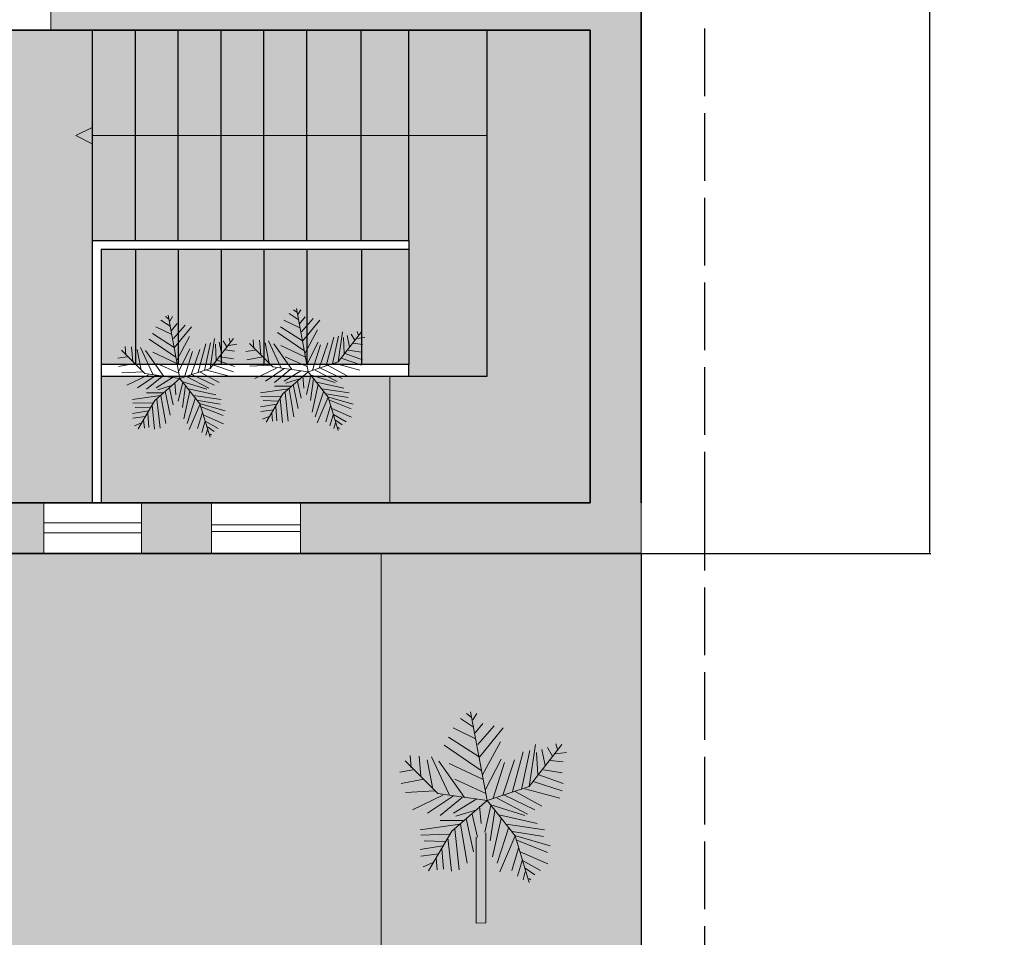
# Model space of a CAD drawing. Units: inches. Extents: x 1316 to 1777, y 813 to 1650.
# Tile 4 of 22: x 1603 to 1777, y 963 to 1126. Entities that reach past the tile are written whole.
import ezdxf

# ---------------------------------------------------------------- set-up
doc = ezdxf.new("R2010")
doc.units = ezdxf.units.IN
doc.header["$MEASUREMENT"] = 0
doc.linetypes.add('ACAD_ISO02W100', pattern=[15, 12, -3])
for name, color, linetype, lineweight in [('A-ANNO-DIMS', 2, 'Continuous', 18), ('A-ANNO-SYMB', 7, 'Continuous', 18), ('A-ANNO-SYMB-PATT', 7, 'Continuous', 13), ('A-FLOR-STRS', 7, 'Continuous', 25), ('A-FLOR-STRS-PATT', 252, 'Continuous', 13), ('A-WALL-PATT', 250, 'Continuous', 13), ('C-PROP', 8, 'ACAD_ISO02W100', 25), ('greenary', 106, 'Continuous', 13), ('L-HRDS', 8, 'Continuous', 18), ('L-HRDS-PATT', 252, 'Continuous', 13), ('L-PLNT-PATT', 74, 'Continuous', 13), ('walls', 250, 'Continuous', 35), ('windows', 141, 'Continuous', 18)]:
    doc.layers.add(name, color=color, linetype=linetype, lineweight=lineweight)
doc.layers.add('A-FLOR-PATT', color=254, linetype='Continuous', lineweight=13, true_color=0xfeeab9)
doc.styles.get("Standard").update_dxf_attribs({"font": 'arial.ttf'})
doc.dimstyles.get("Standard").update_dxf_attribs({"dimtxt": 7, "dimasz": 0.18, "dimexe": 0.18, "dimexo": 0.0625, "dimgap": 0.09, "dimtad": 0, "dimtih": 1, "dimtoh": 1, "dimzin": 0, "dimdsep": 46, "dimlunit": 3, "dimtxsty": 'Standard', "dimcen": 0.09, "dimadec": 0, "dimazin": 0, "dimtfac": 1, "dimtofl": 0, "dimtmove": 0, "dimatfit": 3, "dimfxl": 1, "dimtolj": 1, "dimtzin": 0, "dimarcsym": 0})

# ---------------------------------------------------------------- blocks, each defined once
blk = doc.blocks.new('*U13')
for p, q in [((0, 0), (-10.5, 57)), ((-8.737, 47.138), (-17.069, 52.711)), ((-10.186, 53.64), (-13.084, 55.962)), ((-9.099, 51.782), (-6.563, 55.962)), ((-7.288, 39.707), (-21.778, 46.673)), ((-7.65, 43.423), (-2.578, 49.46)), ((-5.839, 35.992), (4.667, 48.067)), ((-5.114, 27.632), (10.463, 46.673)), ((-5.114, 28.097), (-24.676, 40.636)), ((-3.665, 19.273), (-27.574, 35.527)), ((-2.941, 16.486), (8.652, 37.85)), ((22.055, 7.198), (27.489, 32.277)), ((27, 9), (48, 36)), ((27.127, 9.056), (31.112, 35.992)), ((35.096, 32.741), (37.27, 22.524)), ((38.719, 34.134), (41.979, 28.561)), ((44.153, 36.456), (45.239, 32.741)), ((-31.5, 4.5), (-52.5, 25.5)), ((-48.585, 21.131), (-49.309, 29.026)), ((-43.513, 28.561), (-42.427, 15.558)), ((-38.442, 26.239), (-34.819, 7.663)), ((-35.544, 28.097), (-24.314, 3.947)), ((-14.533, 2.09), (-30.834, 25.31)), ((-1.129, 6.734), (9.014, 26.704)), ((10.101, 3.483), (17.708, 26.239)), ((16.259, 5.805), (23.142, 31.348)), ((31.836, 30.883), (32.561, 16.486)), ((40.53, 25.775), (48.862, 24.846)), ((43.791, 29.954), (51.036, 30.883)), ((-47.498, 19.737), (-55.83, 18.344)), ((-24.314, 23.917), (-2.941, 13.7)), ((3.942, 1.625), (11.187, 24.381)), ((36.183, 19.737), (48.137, 17.88)), ((-40.615, 13.7), (-55.105, 10.913)), ((-20.691, 13.7), (-1.129, 4.876)), ((33.285, 16.486), (48.862, 10.913)), ((0, 0), (27, 9)), ((24.229, 7.663), (46.688, 1.625)), ((29.662, 12.307), (48.137, 6.269)), ((-33.37, 6.269), (-52.207, 5.34)), ((-28.299, 3.483), (-47.86, -5.805)), ((-21.416, 3.018), (-38.079, -8.128)), ((0, 0), (-31.5, 4.5)), ((-15.982, 2.09), (-30.11, -9.521)), ((0, 0), (-22.5, -19.5)), ((-6.563, 1.161), (-21.416, -8.128)), ((0, 0), (18, -22.5)), ((6.478, 1.625), (26.04, -8.592)), ((11.187, 3.483), (30.749, -5.805)), ((18.07, 5.805), (35.096, -3.483)), ((-6.563, -5.805), (-19.967, -9.985)), ((-4.752, -3.483), (-3.665, -14.629)), ((2.493, -3.019), (-1.491, -20.202)), ((1.769, -2.555), (24.229, -9.521)), ((5.029, -6.27), (2.131, -25.775)), ((-13.446, -11.378), (-8.737, -32.741)), ((-9.461, -8.592), (-6.201, -23.453)), ((9.014, -11.378), (3.58, -35.992)), ((7.565, -9.056), (32.198, -14.629)), ((-17.431, -15.094), (-42.789, -18.809)), ((-15.257, -12.772), (-30.11, -12.772)), ((-20.691, -18.345), (-17.793, -44.352)), ((-17.069, -15.094), (-12.721, -40.172)), ((14.085, -16.951), (6.478, -40.172)), ((12.274, -15.094), (36.907, -18.809)), ((-24.314, -21.596), (-42.427, -22.06)), ((-22.5, -19.5), (-37.5, -45)), ((-25.038, -23.918), (-22.865, -45.281)), ((18.07, -22.524), (8.289, -45.745)), ((16.259, -19.738), (36.183, -22.989)), ((18, -22.5), (27, -52.5)), ((18.433, -22.524), (40.53, -29.026)), ((-28.299, -29.026), (-42.789, -31.348)), ((-26.849, -26.24), (-40.253, -25.775)), ((-29.023, -30.884), (-27.936, -43.887)), ((20.244, -30.419), (15.897, -44.816)), ((19.157, -25.311), (38.719, -33.206)), ((-30.834, -34.135), (-42.427, -35.528)), ((-32.646, -36.921), (-31.921, -44.352)), ((22.78, -37.85), (19.519, -48.532)), ((21.331, -32.741), (39.081, -40.636)), ((-34.457, -39.708), (-40.978, -42.494)), ((22.78, -38.314), (34.372, -44.816)), ((24.591, -43.423), (30.749, -47.603)), ((24.591, -45.745), (23.142, -50.854)), ((26.764, -49.925), (28.213, -50.854))]:
    blk.add_line(p, q)
blk = doc.blocks.new('*D50')
at = {"layer": 'A-ANNO-DIMS', "color": 0, "lineweight": -2, "transparency": 16777216}
for p, q in [((1377.06, 1063.81), (1377.06, 817.77)), ((1713.17, 1031.11), (1713.17, 817.77)), ((1377.24, 817.95), (1532.95, 817.95)), ((1712.99, 817.95), (1557.29, 817.95))]:
    blk.add_line(p, q, dxfattribs=at)
at = {"layer": 'A-ANNO-DIMS', "color": 0, "transparency": 16777216}
for points in [[(1377.24, 817.98), (1377.24, 817.92), (1377.06, 817.95)], [(1712.99, 817.98), (1712.99, 817.92), (1713.17, 817.95)]]:
    blk.add_solid(points, dxfattribs=at)
at = {"layer": 'Defpoints', "color": 0, "transparency": 16777216}
for p in [(1377.06, 1063.87), (1713.17, 1031.17), (1713.17, 817.95)]:
    blk.add_point(p, dxfattribs=at)
at = {"layer": 'A-ANNO-DIMS', "color": 0, "transparency": 16777216, "insert": (1545.12, 817.95), "char_height": 7, "attachment_point": 5}
blk.add_mtext('\\A1;28\'-0"', dxfattribs=at)
blk = doc.blocks.new('*D51')
at = {"layer": 'A-ANNO-DIMS', "color": 0, "lineweight": -2, "transparency": 16777216}
for p, q in [((1713.24, 1575.37), (1764.48, 1575.37)), ((1764.3, 1575.19), (1764.3, 1306.92)), ((1764.3, 1031.35), (1764.3, 1299.62)), ((1713.24, 1031.17), (1764.48, 1031.17))]:
    blk.add_line(p, q, dxfattribs=at)
at = {"layer": 'A-ANNO-DIMS', "color": 0, "transparency": 16777216}
for points in [[(1764.27, 1575.19), (1764.33, 1575.19), (1764.3, 1575.37)], [(1764.27, 1031.35), (1764.33, 1031.35), (1764.3, 1031.17)]]:
    blk.add_solid(points, dxfattribs=at)
at = {"layer": 'Defpoints', "color": 0, "transparency": 16777216}
for p in [(1713.17, 1575.37), (1764.3, 1575.37), (1713.17, 1031.17)]:
    blk.add_point(p, dxfattribs=at)
at = {"layer": 'A-ANNO-DIMS', "color": 0, "transparency": 16777216, "insert": (1764.3, 1303.27), "char_height": 7, "attachment_point": 5}
blk.add_mtext('\\A1;45\'-4"', dxfattribs=at)

msp = doc.modelspace()

# ---------------------------------------------------------------- hatches: boundary and pattern name
at = {"layer": 'A-ANNO-SYMB-PATT'}
h = msp.add_hatch(color=256, dxfattribs=at)
h.dxf.hatch_style = 1
h.paths.add_polyline_path([(1613.066, 1105.235), (1616.06, 1103.693), (1616.06, 1105.253), (1616.06, 1106.696)])
at = {"layer": 'A-FLOR-PATT'}
h = msp.add_hatch(color=256, dxfattribs=at)
h.dxf.hatch_style = 1
h.paths.add_polyline_path([(1567.673, 1281.369), (1651.673, 1281.369), (1651.673, 1365.369), (1597.673, 1365.369), (1597.673, 1429.869), (1570.345, 1429.869), (1570.345, 1471.869), (1510.345, 1471.869), (1510.345, 1429.869), (1444.564, 1429.869), (1444.564, 1322.882), (1444.564, 1300.088), (1510.564, 1300.088), (1510.564, 1295.094), (1510.564, 1240.869), (1386.064, 1240.869), (1386.064, 1171.185), (1400.961, 1171.185), (1400.961, 1106.742), (1386.064, 1106.742), (1386.064, 1072.869), (1510.564, 1072.869), (1510.564, 1040.173), (1541.068, 1040.173, -0.367085), (1572.764, 1069.547), (1572.764, 1069.579), (1574.225, 1069.579), (1574.225, 1040.173), (1616.037, 1040.173), (1616.037, 1086.627), (1616.037, 1103.705), (1613.066, 1105.235), (1616.037, 1106.686), (1616.037, 1123.869), (1567.673, 1123.869)])
h.paths.add_polyline_path([(1508.987, 1198.018), (1511.117, 1198.018), (1511.117, 1200.148), (1532.595, 1200.148), (1532.595, 1198.018), (1534.725, 1198.018), (1534.725, 1176.008), (1530.465, 1176.008), (1530.465, 1176.718), (1513.247, 1176.718), (1513.247, 1176.008), (1508.987, 1176.008)], flags=16)
h.paths.add_polyline_path([(1505.979, 1151.315), (1521.504, 1151.315), (1521.504, 1123.623), (1505.979, 1123.623)], flags=16)
h.paths.add_polyline_path([(1507.734, 1150.101, -1), (1506.932, 1150.101, -1)], flags=0)
h.paths.add_polyline_path([(1512.288, 1138.353), (1512.28, 1138.392), (1512.219, 1138.376)], flags=0)
h.paths.add_polyline_path([(1511.539, 1138.926), (1511.802, 1138.967), (1511.817, 1139.27), (1511.607, 1139.246)], flags=0)
h.paths.add_polyline_path([(1513.745, 1140.234), (1513.68, 1139.885), (1514.014, 1140.045), (1513.855, 1140.308)], flags=0)
h.paths.add_polyline_path([(1513.759, 1139.089), (1514.005, 1139.255), (1513.807, 1139.483), (1513.564, 1139.327)], flags=0)
h.paths.add_polyline_path([(1514.219, 1138.385), (1514.336, 1138.33), (1514.544, 1138.32), (1514.802, 1138.874), (1514.451, 1138.716)], flags=0)
h.paths.add_polyline_path([(1514.577, 1137.439), (1514.573, 1137.4), (1514.699, 1137.4), (1514.696, 1137.402)], flags=0)
h.paths.add_polyline_path([(1512.26, 1136.199), (1512.199, 1136.399), (1512.032, 1136.325), (1512.095, 1136.101), (1512.257, 1136.192)], flags=0)
h.paths.add_polyline_path([(1512.644, 1137.274), (1512.356, 1137.23), (1512.432, 1137.049), (1512.703, 1137.093)], flags=0)
h.paths.add_polyline_path([(1513.049, 1137.593), (1512.979, 1137.8), (1512.843, 1137.757), (1512.887, 1137.556)], flags=0)
h.paths.add_polyline_path([(1513.269, 1138.556), (1513.571, 1137.962), (1513.459, 1136.814), (1513.212, 1137.878), (1513.032, 1138.443)], flags=0)
h.paths.add_polyline_path([(1514.891, 1136.377), (1514.696, 1136.401), (1514.683, 1136.246), (1514.87, 1136.165)], flags=0)
h.paths.add_polyline_path([(1514.142, 1137.293), (1514.047, 1136.743), (1514.27, 1136.751), (1514.328, 1137.265)], flags=0)
h.paths.add_polyline_path([(1515.362, 1138.976), (1515.334, 1138.638), (1515.596, 1138.588), (1515.627, 1138.932)], flags=0)
h.paths.add_polyline_path([(1537.285, 1177.912), (1537.995, 1177.912), (1537.995, 1195.13), (1537.285, 1195.13), (1537.285, 1199.39), (1559.295, 1199.39), (1559.295, 1197.26), (1561.425, 1197.26), (1561.425, 1175.782), (1559.295, 1175.782), (1559.295, 1173.652), (1559.379, 1173.652), (1559.379, 1171.514), (1561.517, 1171.514), (1561.517, 1098.819), (1559.379, 1098.819), (1559.379, 1096.68), (1537.285, 1096.68), (1537.285, 1100.957), (1537.997, 1100.957), (1537.997, 1169.376), (1537.285, 1169.376), (1537.285, 1173.652)], flags=16)
h.paths.add_polyline_path([(1518.623, 1345.565), (1519.133, 1345.48), (1519.133, 1345.485), (1518.623, 1345.567)], flags=16)
h.paths.add_polyline_path([(1518.798, 1374.15), (1519.308, 1374.064), (1519.308, 1374.069), (1518.798, 1374.152)], flags=16)
h.paths.add_polyline_path([(1537.764, 1413.501), (1537.678, 1412.991), (1537.683, 1412.991), (1537.766, 1413.501)], flags=16)
h.paths.add_polyline_path([(1572.905, 1373.821), (1573.927, 1373.975), (1574.027, 1390.309), (1573.007, 1390.475), (1573.007, 1390.475)], flags=16)
h.paths.add_polyline_path([(1572.73, 1345.237), (1573.752, 1345.39), (1573.852, 1361.724), (1572.832, 1361.89), (1572.832, 1361.89)], flags=16)
h.paths.add_polyline_path([(1537.211, 1322.643), (1537.364, 1321.621), (1553.698, 1321.521), (1553.864, 1322.541)], flags=16)
h.paths.add_polyline_path([(1535.908, 1331.328), (1527.214, 1331.382), (1527.664, 1404.885), (1564.416, 1404.66), (1563.966, 1331.157), (1555.273, 1331.21), (1553.947, 1323.051), (1537.134, 1323.154)], flags=16)
h.paths.add_polyline_path([(1536.15, 1336.503), (1536.235, 1337.572), (1536.323, 1338.628), (1536.411, 1339.663), (1536.495, 1340.67), (1536.574, 1341.66), (1536.648, 1342.648), (1536.717, 1343.649), (1536.78, 1344.678), (1536.837, 1345.75), (1536.913, 1347.475), (1536.93, 1348.082), (1536.867, 1346.314), (1536.754, 1344.188), (1536.619, 1342.219), (1536.495, 1340.67), (1536.411, 1339.663), (1536.323, 1338.628), (1536.235, 1337.572), (1536.15, 1336.503), (1536.071, 1335.432), (1536.002, 1334.37), (1535.917, 1332.754), (1535.909, 1332.308), (1535.964, 1333.78), (1536.071, 1335.432)], flags=0)
h.paths.add_polyline_path([(1540.412, 1338.345), (1540.539, 1339.037), (1540.667, 1339.758), (1540.798, 1340.518), (1540.93, 1341.325), (1541.063, 1342.187), (1541.196, 1343.109), (1541.326, 1344.085), (1541.45, 1345.102), (1541.566, 1346.15), (1541.669, 1347.219), (1541.758, 1348.296), (1541.829, 1349.371), (1541.879, 1350.434), (1541.906, 1351.476), (1541.91, 1352.5), (1541.895, 1353.512), (1541.861, 1354.518), (1541.812, 1355.524), (1541.749, 1356.537), (1541.674, 1357.561), (1541.551, 1359.062), (1541.495, 1359.67), (1541.589, 1358.603), (1541.721, 1356.977), (1541.846, 1354.98), (1541.912, 1352.982), (1541.903, 1350.951), (1541.806, 1348.87), (1541.628, 1346.713), (1541.396, 1344.612), (1541.135, 1342.656), (1540.872, 1340.947), (1540.617, 1339.466), (1540.412, 1338.345), (1540.288, 1337.675), (1540.166, 1337.018), (1540.049, 1336.365), (1539.937, 1335.71), (1539.837, 1335.055), (1539.758, 1334.403), (1539.709, 1333.756), (1539.697, 1333.12), (1539.751, 1332.162), (1539.822, 1331.89), (1539.691, 1332.775), (1539.714, 1334.035), (1539.867, 1335.303), (1540.085, 1336.577), (1540.288, 1337.675)], flags=0)
h.paths.add_polyline_path([(1545.599, 1331.584), (1545.601, 1331.617), (1545.614, 1331.689), (1545.737, 1332.197), (1545.767, 1332.332), (1545.84, 1332.681), (1545.925, 1333.114), (1546.016, 1333.614), (1546.108, 1334.164), (1546.196, 1334.748), (1546.276, 1335.349), (1546.342, 1335.952), (1546.388, 1336.539), (1546.412, 1337.098), (1546.414, 1337.632), (1546.395, 1338.145), (1546.359, 1338.645), (1546.306, 1339.137), (1546.24, 1339.627), (1546.161, 1340.121), (1546.073, 1340.625), (1545.888, 1341.63), (1545.718, 1342.621), (1545.547, 1343.945), (1545.432, 1345.534), (1545.404, 1347.402), (1545.418, 1348.013), (1545.411, 1346.957), (1545.425, 1345.988), (1545.463, 1345.105), (1545.521, 1344.301), (1545.596, 1343.566), (1545.683, 1342.892), (1545.778, 1342.27), (1545.877, 1341.691), (1545.977, 1341.145), (1546.133, 1340.297), (1546.327, 1339.075), (1546.434, 1337.615), (1546.377, 1336.279), (1546.246, 1335.079), (1546.032, 1333.665), (1545.84, 1332.681), (1545.767, 1332.332)], flags=0)
h.paths.add_polyline_path([(1551.803, 1337.656), (1551.963, 1338.25), (1552.102, 1338.801), (1552.225, 1339.338), (1552.331, 1339.865), (1552.418, 1340.377), (1552.487, 1340.873), (1552.536, 1341.348), (1552.563, 1341.801), (1552.569, 1342.228), (1552.551, 1342.627), (1552.51, 1342.995), (1552.446, 1343.333), (1552.363, 1343.646), (1552.261, 1343.937), (1552.144, 1344.207), (1552.012, 1344.461), (1551.868, 1344.7), (1551.746, 1344.882), (1550.887, 1346.052), (1550.428, 1347.126), (1550.183, 1348.353), (1550.048, 1349.632), (1549.978, 1351.224), (1549.974, 1353.141), (1549.989, 1353.748), (1549.975, 1352.682), (1549.977, 1351.708), (1549.996, 1350.825), (1550.031, 1350.027), (1550.082, 1349.31), (1550.15, 1348.669), (1550.234, 1348.098), (1550.335, 1347.593), (1550.452, 1347.149), (1550.584, 1346.76), (1550.73, 1346.419), (1550.887, 1346.117), (1551.05, 1345.848), (1551.217, 1345.602), (1551.386, 1345.372), (1551.553, 1345.151), (1552, 1344.537), (1552.454, 1343.495), (1552.591, 1342.266), (1552.509, 1340.905), (1552.246, 1339.367), (1551.925, 1338.101), (1551.619, 1336.984), (1551.406, 1336.2), (1551.01, 1334.699), (1550.877, 1334.155), (1551.264, 1335.677), (1551.619, 1336.984)], flags=0)
h.paths.add_polyline_path([(1558.642, 1348.348), (1558.795, 1348.811), (1558.918, 1349.215), (1559.008, 1349.575), (1559.061, 1349.904), (1559.076, 1350.214), (1559.054, 1350.506), (1559.001, 1350.776), (1558.919, 1351.021), (1558.814, 1351.239), (1558.688, 1351.425), (1558.546, 1351.578), (1558.392, 1351.694), (1558.229, 1351.772), (1558.059, 1351.812), (1557.882, 1351.819), (1557.701, 1351.794), (1557.515, 1351.742), (1557.327, 1351.665), (1557.136, 1351.566), (1556.944, 1351.448), (1556.752, 1351.315), (1556.742, 1351.307), (1556.175, 1350.878), (1555.982, 1350.741), (1555.79, 1350.618), (1555.103, 1350.248), (1554.019, 1350.696), (1553.658, 1351.734), (1553.592, 1352.861), (1553.705, 1354.248), (1553.753, 1354.657), (1553.685, 1354.004), (1553.638, 1353.425), (1553.615, 1352.918), (1553.615, 1352.476), (1553.637, 1352.094), (1553.681, 1351.766), (1553.745, 1351.485), (1553.828, 1351.246), (1553.929, 1351.043), (1554.048, 1350.87), (1554.182, 1350.722), (1554.33, 1350.599), (1554.491, 1350.501), (1554.662, 1350.43), (1554.841, 1350.388), (1555.026, 1350.374), (1555.215, 1350.39), (1555.406, 1350.437), (1555.598, 1350.514), (1555.79, 1350.618), (1555.982, 1350.741), (1556.175, 1350.878), (1556.367, 1351.024), (1556.559, 1351.171), (1556.752, 1351.315), (1556.944, 1351.448), (1557.136, 1351.566), (1557.327, 1351.665), (1558.043, 1351.957), (1558.894, 1351.316), (1559.137, 1350.09), (1558.886, 1349.087), (1558.642, 1348.348), (1558.463, 1347.812), (1558.261, 1347.187), (1558.039, 1346.459), (1557.677, 1345.175), (1557.549, 1344.636), (1557.909, 1346.03), (1558.329, 1347.408)], flags=0)
h.paths.add_polyline_path([(1562.145, 1353.919), (1562.25, 1354.68), (1562.341, 1355.344), (1562.416, 1355.924), (1562.475, 1356.431), (1562.518, 1356.872), (1562.544, 1357.254), (1562.554, 1357.582), (1562.548, 1357.862), (1562.525, 1358.1), (1562.486, 1358.303), (1562.432, 1358.476), (1562.361, 1358.624), (1562.277, 1358.748), (1562.18, 1358.848), (1562.073, 1358.925), (1561.958, 1358.977), (1561.837, 1359.006), (1561.711, 1359.011), (1561.584, 1358.992), (1561.456, 1358.949), (1561.342, 1358.895), (1560.78, 1358.554), (1560.631, 1358.473), (1560.474, 1358.403), (1560.311, 1358.348), (1559.637, 1358.207), (1558.973, 1358.904), (1558.816, 1360.002), (1558.804, 1361.236), (1558.83, 1361.674), (1558.807, 1360.917), (1558.813, 1360.297), (1558.845, 1359.795), (1558.902, 1359.397), (1558.982, 1359.087), (1559.082, 1358.849), (1559.2, 1358.666), (1559.334, 1358.525), (1559.482, 1358.421), (1559.639, 1358.351), (1559.804, 1358.311), (1559.973, 1358.3), (1560.143, 1358.313), (1560.311, 1358.348), (1560.474, 1358.403), (1560.631, 1358.473), (1560.78, 1358.554), (1560.923, 1358.641), (1561.061, 1358.729), (1561.196, 1358.813), (1561.382, 1358.92), (1561.342, 1358.895), (1561.972, 1359.194), (1562.536, 1358.367), (1562.56, 1357.311), (1562.455, 1356.226), (1562.323, 1355.206), (1562.145, 1353.919), (1562.026, 1353.049), (1561.815, 1351.457), (1561.752, 1350.933), (1561.948, 1352.479)], flags=0)
h.paths.add_polyline_path([(1572.764, 1069.547, 0.367085), (1541.068, 1040.173), (1572.764, 1040.173)], flags=17)
h.paths.add_polyline_path([(1572.764, 1040.173), (1541.068, 1040.173, 0.0299535), (1540.829, 1036.182), (1540.829, 1031.173), (1574.225, 1031.173), (1574.225, 1036.182), (1572.764, 1036.182)])
at = {"layer": 'A-FLOR-STRS-PATT'}
h = msp.add_hatch(color=256, dxfattribs=at)
h.dxf.hatch_style = 1
h.paths.add_polyline_path([(1623.621, 1105.248), (1616.037, 1105.248), (1616.037, 1086.627), (1623.621, 1086.627)])
h.paths.add_polyline_path([(1623.621, 1123.869), (1616.037, 1123.869), (1616.037, 1105.248), (1623.621, 1105.248)])
h.paths.add_polyline_path([(1631.206, 1105.248), (1623.621, 1105.248), (1623.621, 1086.627), (1631.206, 1086.627)])
h.paths.add_polyline_path([(1631.206, 1123.869), (1623.621, 1123.869), (1623.621, 1105.248), (1631.206, 1105.248)])
h.paths.add_polyline_path([(1638.79, 1105.248), (1631.206, 1105.248), (1631.206, 1086.627), (1638.79, 1086.627)])
h.paths.add_polyline_path([(1638.79, 1123.869), (1631.206, 1123.869), (1631.206, 1105.248), (1638.79, 1105.248)])
h.paths.add_polyline_path([(1646.374, 1105.248), (1638.79, 1105.248), (1638.79, 1086.627), (1646.374, 1086.627)])
h.paths.add_polyline_path([(1646.374, 1123.869), (1638.79, 1123.869), (1638.79, 1105.248), (1646.374, 1105.248)])
h.paths.add_polyline_path([(1653.958, 1105.248), (1646.374, 1105.248), (1646.374, 1086.627), (1653.958, 1086.627)])
h.paths.add_polyline_path([(1653.958, 1123.869), (1646.374, 1123.869), (1646.374, 1105.248), (1653.958, 1105.248)])
h.paths.add_polyline_path([(1663.586, 1105.248), (1653.958, 1105.248), (1653.958, 1086.627), (1663.586, 1086.627)])
h.paths.add_polyline_path([(1663.586, 1123.869), (1653.958, 1123.869), (1653.958, 1105.248), (1663.586, 1105.248)])
h.paths.add_polyline_path([(1672.026, 1105.248), (1663.586, 1105.248), (1663.586, 1086.627), (1672.026, 1086.627)])
h.paths.add_polyline_path([(1672.026, 1123.869), (1663.586, 1123.869), (1663.586, 1105.248), (1672.026, 1105.248)])
h = msp.add_hatch(color=256, dxfattribs=at)
h.dxf.hatch_style = 1
h.paths.add_polyline_path([(1685.903, 1105.248), (1672.026, 1105.248), (1672.026, 1086.627), (1672.026, 1085.053), (1672.026, 1064.656), (1672.026, 1062.613), (1685.903, 1062.613)])
h.paths.add_polyline_path([(1685.903, 1123.869), (1672.026, 1123.869), (1672.026, 1105.248), (1685.903, 1105.248)])
h = msp.add_hatch(color=256, dxfattribs=at)
h.dxf.hatch_style = 1
h.paths.add_polyline_path([(1623.621, 1085.053), (1617.549, 1085.053), (1617.549, 1064.656), (1623.621, 1064.656)])
h.paths.add_polyline_path([(1631.206, 1085.053), (1623.621, 1085.053), (1623.621, 1064.656), (1631.206, 1064.656)])
h.paths.add_polyline_path([(1638.79, 1085.053), (1631.206, 1085.053), (1631.206, 1064.656), (1638.79, 1064.656)])
h.paths.add_polyline_path([(1646.374, 1085.053), (1638.79, 1085.053), (1638.79, 1064.656), (1646.374, 1064.656)])
h.paths.add_polyline_path([(1653.958, 1085.053), (1646.374, 1085.053), (1646.374, 1064.656), (1653.958, 1064.656)])
h.paths.add_polyline_path([(1663.648, 1085.053), (1653.958, 1085.053), (1653.958, 1064.656), (1663.648, 1064.656)])
h.paths.add_polyline_path([(1672.026, 1085.053), (1663.648, 1085.053), (1663.648, 1064.656), (1672.026, 1064.656)])
at = {"layer": 'A-WALL-PATT'}
h = msp.add_hatch(color=256, dxfattribs=at)
h.dxf.hatch_style = 1
h.paths.add_polyline_path([(1713.173, 1281.369), (1656.173, 1281.369), (1656.173, 1298.258), (1651.673, 1298.258), (1651.673, 1281.369), (1567.673, 1281.369), (1567.673, 1266.995), (1572.173, 1266.995), (1572.173, 1276.869), (1704.173, 1276.869), (1704.173, 1132.869), (1608.64, 1132.869), (1608.64, 1123.869), (1704.173, 1123.869), (1704.173, 1040.173), (1652.869, 1040.173), (1652.869, 1031.173), (1713.173, 1031.173), (1713.173, 1040.173)])
h.paths.add_polyline_path([(1572.173, 1237.955), (1567.673, 1237.955), (1567.673, 1123.869), (1583.146, 1123.869), (1583.146, 1132.869), (1572.173, 1132.869)], flags=17)
h.paths.add_polyline_path([(1510.345, 1566.369), (1524.171, 1566.369), (1524.171, 1571.985), (1524.171, 1575.369), (1445.955, 1575.369), (1445.955, 1566.369), (1505.845, 1566.369), (1505.845, 1469.591), (1510.345, 1469.591), (1510.345, 1471.869), (1529.081, 1471.869), (1529.081, 1476.369), (1510.345, 1476.369)])
h.paths.add_polyline_path([(1609.722, 1575.369), (1545.119, 1575.369), (1545.119, 1566.369), (1570.345, 1566.369), (1570.345, 1476.369), (1562.477, 1476.369), (1562.477, 1471.869), (1570.345, 1471.869), (1570.345, 1469.591), (1574.845, 1469.591), (1574.845, 1566.369), (1609.722, 1566.369)])
h.paths.add_polyline_path([(1713.173, 1575.369), (1655.233, 1575.369), (1655.233, 1566.369), (1704.173, 1566.369), (1704.173, 1434.369), (1574.845, 1434.369), (1574.845, 1440.551), (1574.701, 1440.551), (1570.345, 1440.551), (1570.345, 1429.869), (1597.673, 1429.869), (1597.673, 1408.281), (1602.173, 1408.281), (1602.173, 1429.869), (1704.173, 1429.869), (1704.173, 1410.704), (1707.375, 1410.704), (1713.173, 1410.704)])
h.paths.add_polyline_path([(1713.173, 1383.676), (1704.173, 1383.676), (1704.173, 1369.869), (1602.173, 1369.869), (1602.173, 1379.241), (1597.673, 1379.241), (1597.673, 1365.369), (1713.173, 1365.369)])
h.paths.add_polyline_path([(1444.564, 1429.869), (1510.345, 1429.869), (1510.345, 1440.551), (1505.845, 1440.551), (1505.845, 1434.369), (1386.064, 1434.369), (1386.064, 1566.369), (1400.445, 1566.369), (1400.445, 1575.369), (1377.064, 1575.369), (1377.064, 1412.813), (1380.509, 1412.813), (1386.064, 1412.813), (1386.064, 1429.869), (1440.064, 1429.869), (1440.064, 1401.229), (1444.564, 1401.229)])
h.paths.add_polyline_path([(1444.564, 1372.189), (1440.064, 1372.189), (1440.064, 1369.869), (1386.064, 1369.869), (1386.064, 1378.758), (1377.064, 1378.758), (1377.064, 1349.201), (1381.118, 1349.201), (1386.064, 1349.201), (1386.064, 1365.369), (1440.064, 1365.369), (1440.064, 1322.882), (1444.564, 1322.882)])
h.paths.add_polyline_path([(1510.564, 1295.094), (1506.064, 1295.094), (1506.064, 1245.369), (1386.064, 1245.369), (1386.064, 1272.582), (1377.064, 1272.582), (1377.064, 1212.905), (1380.1, 1212.905), (1386.064, 1212.905), (1386.064, 1240.869), (1510.564, 1240.869)])
h.paths.add_polyline_path([(1386.064, 1163.761), (1377.064, 1163.761), (1377.064, 1063.869), (1419.363, 1063.869), (1419.363, 1072.869), (1386.064, 1072.869)])
h.paths.add_polyline_path([(1510.564, 1072.869), (1469.381, 1072.869), (1469.381, 1063.869), (1501.564, 1063.869), (1501.564, 1033.023), (1501.564, 1031.173), (1540.829, 1031.173), (1540.829, 1036.182, -0.0299535), (1541.068, 1040.173), (1510.564, 1040.173)])
h.paths.add_polyline_path([(1607.369, 1040.173), (1574.225, 1040.173), (1574.225, 1036.182), (1574.225, 1031.173), (1607.369, 1031.173)], flags=17)
h.paths.add_polyline_path([(1637.054, 1040.173), (1624.706, 1040.173), (1624.706, 1031.173), (1637.054, 1031.173)], flags=17)
at = {"layer": 'L-HRDS-PATT'}
h = msp.add_hatch(color=256, dxfattribs=at)
h.dxf.hatch_style = 1
h.paths.add_polyline_path([(1492.539, 953.689), (1377.064, 953.689), (1365.834, 953.689), (1365.735, 922.018), (1492.539, 922.018)])
h.paths.add_polyline_path([(1724.399, 953.689), (1713.173, 953.689), (1606.561, 953.689), (1606.561, 922.018), (1724.399, 922.018)])
h.paths.add_polyline_path([(1667.146, 959.936), (1596.428, 959.936), (1596.428, 953.689), (1604.517, 953.689), (1604.517, 955.706), (1606.561, 955.706), (1606.561, 953.689), (1667.146, 953.689)])
h.paths.add_polyline_path([(1704.173, 1123.869), (1685.903, 1123.869), (1685.903, 1062.613), (1672.026, 1062.613), (1668.679, 1062.613), (1668.679, 1040.173), (1704.173, 1040.173)])
h = msp.add_hatch(color=256, dxfattribs=at)
h.dxf.hatch_style = 1
h.paths.add_polyline_path([(1667.146, 1031.173), (1596.428, 1031.173), (1596.428, 982.68), (1596.428, 971.474), (1596.428, 959.936), (1667.146, 959.936)])
h = msp.add_hatch(color=256, dxfattribs=at)
h.dxf.hatch_style = 1
h.paths.add_polyline_path([(1713.173, 1031.173), (1667.146, 1031.173), (1667.146, 953.689), (1713.173, 953.689)])
at = {"layer": 'L-PLNT-PATT'}
h = msp.add_hatch(color=256, dxfattribs=at)
h.dxf.hatch_style = 1
h.paths.add_polyline_path([(1501.564, 1031.173), (1501.564, 1033.023), (1501.564, 1063.869), (1386.064, 1063.869), (1386.064, 965.355), (1501.564, 965.355)])
h.paths.add_polyline_path([(1668.679, 1062.613), (1617.549, 1062.613), (1617.549, 1040.173), (1624.706, 1040.173), (1668.679, 1040.173)])

# ---------------------------------------------------------------- linework, layer by layer
at = {"layer": 'A-ANNO-SYMB'}
for p, q in [((1616.06, 1106.696), (1613.066, 1105.235)), ((1613.066, 1105.235), (1616.06, 1103.693)), ((1616.037, 1105.248), (1685.903, 1105.248))]:
    msp.add_line(p, q, dxfattribs=at)
at = {"layer": 'A-FLOR-STRS'}
for p, q in [((1616.037, 1086.627), (1616.037, 1123.869)), ((1623.621, 1086.627), (1623.621, 1123.869)), ((1631.206, 1086.627), (1631.206, 1123.869)), ((1638.79, 1086.627), (1638.79, 1123.869)), ((1646.374, 1086.627), (1646.374, 1123.869)), ((1653.958, 1086.627), (1653.958, 1123.869)), ((1663.586, 1086.627), (1663.586, 1123.869)), ((1672.026, 1086.627), (1672.026, 1123.869)), ((1685.903, 1062.613), (1685.903, 1123.869)), ((1616.037, 1040.173), (1616.037, 1086.627)), ((1616.037, 1086.627), (1672.026, 1086.627)), ((1672.026, 1086.627), (1672.026, 1085.053)), ((1672.026, 1085.053), (1617.549, 1085.053)), ((1617.549, 1085.053), (1617.549, 1040.173)), ((1623.621, 1085.053), (1623.621, 1064.656)), ((1631.206, 1085.053), (1631.206, 1064.656)), ((1638.79, 1085.053), (1638.79, 1064.656)), ((1646.374, 1085.053), (1646.374, 1064.656)), ((1653.958, 1085.053), (1653.958, 1064.656)), ((1663.648, 1085.053), (1663.648, 1064.656)), ((1672.026, 1085.053), (1672.026, 1064.656)), ((1672.026, 1064.656), (1617.549, 1064.656)), ((1672.026, 1062.613), (1672.026, 1064.656)), ((1617.549, 1062.613), (1672.026, 1062.613)), ((1672.026, 1062.613), (1685.903, 1062.613))]:
    msp.add_line(p, q, dxfattribs=at)
at = {"layer": 'C-PROP'}
for p, q in [((1724.399, 1604.173), (1724.399, 1040.173)), ((1724.399, 1040.173), (1724.399, 953.689))]:
    msp.add_line(p, q, dxfattribs=at)
at = {"layer": 'greenary'}
for p, q in [((1683.94, 980.888), (1683.94, 965.655)), ((1685.699, 965.741), (1685.699, 981.679)), ((1683.94, 965.655), (1685.699, 965.741))]:
    msp.add_line(p, q, dxfattribs=at)
at = {"layer": 'L-HRDS'}
for p, q in [((1668.679, 1062.613), (1668.679, 1040.173)), ((1713.173, 953.689), (1713.173, 1040.173)), ((1667.146, 1031.173), (1667.146, 953.689))]:
    msp.add_line(p, q, dxfattribs=at)
at = {"layer": 'walls'}
for p, q in [((1713.173, 1575.369), (1713.173, 1040.173)), ((1567.673, 1123.869), (1704.173, 1123.869)), ((1704.173, 1123.869), (1704.173, 1040.173)), ((1510.564, 1040.173), (1704.173, 1040.173)), ((1713.173, 1031.173), (1501.564, 1031.173))]:
    msp.add_line(p, q, dxfattribs=at)
at = {"layer": 'windows'}
for p, q in [((1608.64, 1123.869), (1608.64, 1132.869)), ((1583.146, 1123.869), (1608.64, 1123.869)), ((1607.369, 1040.173), (1607.369, 1031.173)), ((1624.706, 1040.173), (1607.369, 1040.173)), ((1607.369, 1040.173), (1607.369, 1036.58)), ((1624.706, 1031.173), (1624.706, 1040.173)), ((1637.054, 1040.173), (1637.054, 1031.173)), ((1652.869, 1040.173), (1637.054, 1040.173)), ((1637.054, 1040.173), (1637.054, 1036.275)), ((1652.869, 1031.173), (1652.869, 1040.173)), ((1607.369, 1036.58), (1624.706, 1036.58)), ((1624.706, 1036.58), (1624.706, 1034.832)), ((1637.054, 1036.275), (1652.869, 1036.275)), ((1652.869, 1036.275), (1652.869, 1035.09)), ((1624.706, 1034.832), (1607.369, 1034.832)), ((1652.869, 1035.09), (1637.054, 1035.09)), ((1607.369, 1031.173), (1624.706, 1031.173)), ((1637.054, 1031.173), (1652.869, 1031.173))]:
    msp.add_line(p, q, dxfattribs=at)

# ---------------------------------------------------------------- block references
at = {"layer": 'greenary'}
for p, xscale, yscale, zscale in [((1654.181, 1063.329), 0.1970946241996355, 0.1970946241996355, 0.1970946241996355), ((1631.499, 1062.146), 0.1970946241996355, 0.1970946241996355, 0.1970946241996355), ((1685.877, 987.384), 0.2760751436618833, 0.2760751436618833, 0.2760751436618833)]:
    msp.add_blockref('*U13', p, dxfattribs=dict(at, xscale=xscale, yscale=yscale, zscale=zscale))

# ---------------------------------------------------------------- dimensions: what is measured, and where the dimension line sits
at = {"layer": 'A-ANNO-DIMS'}
dim = msp.add_linear_dim(base=(1764.299, 1575.369), p1=(1713.173, 1031.173), p2=(1713.173, 1575.369), angle=90, dimstyle='Standard', override={"dimdec": 1, "dimlfac": 1, "dimrnd": 0, "dimzin": 1, "dimdsep": 46, "dimlunit": 4, "dimfrac": 2}, dxfattribs=at)
dim.commit()
dim.dimension.update_dxf_attribs({"geometry": '*D51', "text_midpoint": (1764.299, 1303.271)})
dim = msp.add_linear_dim(base=(1713.173, 817.949), p1=(1377.064, 1063.869), p2=(1713.173, 1031.173), dimstyle='Standard', override={"dimdec": 1, "dimlfac": 1, "dimrnd": 0, "dimzin": 1, "dimdsep": 46, "dimlunit": 4, "dimfrac": 2}, dxfattribs=at)
dim.commit()
dim.dimension.update_dxf_attribs({"geometry": '*D50', "text_midpoint": (1545.119, 817.949)})

doc.saveas('drawing.dxf')
